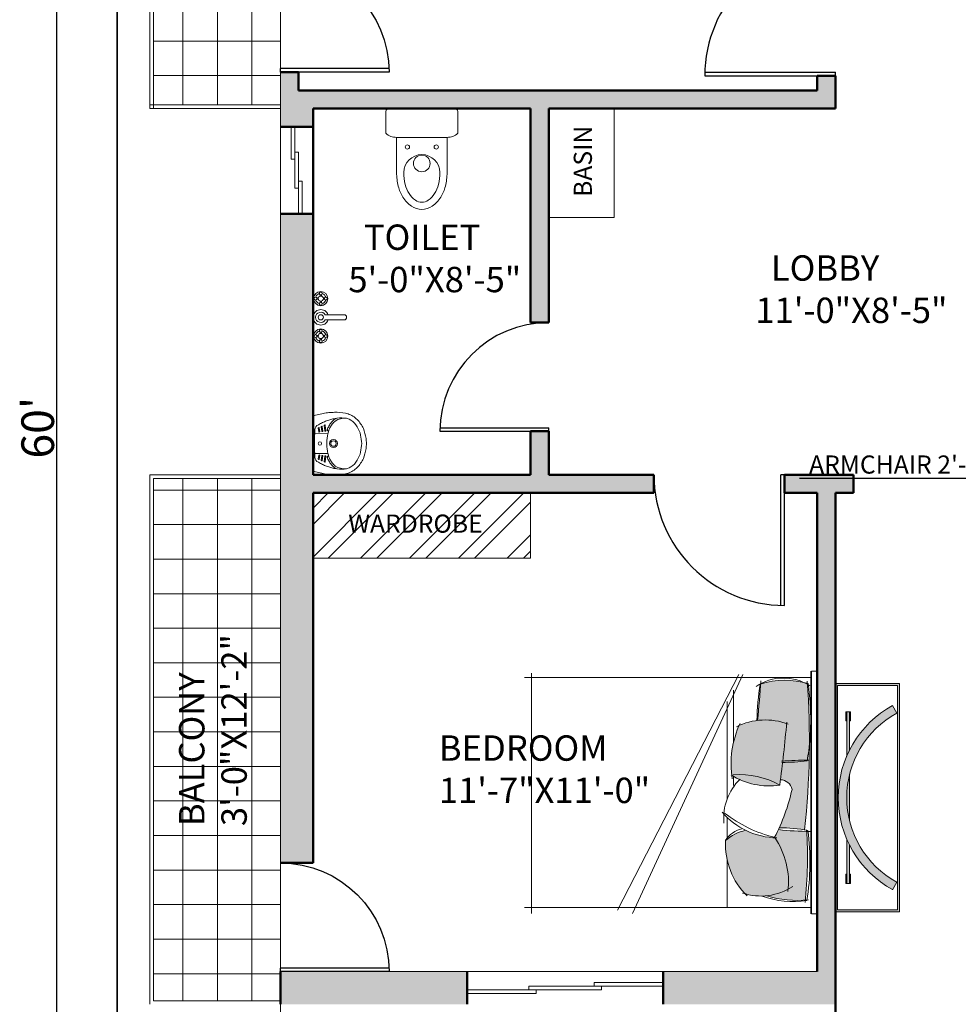
# Model space of a CAD drawing. Units: inches. Extents: x 1734 to 4011, y 1071 to 1891.
# Tile 25 of 27: x 3583 to 3842, y 1313 to 1584. Entities that reach past the tile are written whole.
import ezdxf

# ---------------------------------------------------------------- set-up
doc = ezdxf.new("R2010")
doc.units = ezdxf.units.IN
for name, color, linetype, lineweight in [('0.10', 252, 'Continuous', 9), ('0.15', 34, 'Continuous', 15), ('A-ANNO-DIMS', 2, 'Continuous', 18), ('A-AREA-IDEN', 3, 'Continuous', 18), ('A-DOOR', 3, 'Continuous', 25), ('A-FLOR-FIXT', 9, 'Continuous', 18), ('A-FLOR-PATT', 252, 'Continuous', 13), ('A-FURN', 8, 'Continuous', 18), ('A-FURN-PATT', 252, 'Continuous', 13), ('A-GLAZ', 4, 'Continuous', 18), ('A-WALL', 7, 'Continuous', 50), ('A-WALL-PATT', 8, 'Continuous', 13), ('aparador', 36, 'Continuous', 9), ('C-PROP', 1, 'Continuous', 35), ('moveis', 254, 'Continuous', 5)]:
    doc.layers.add(name, color=color, linetype=linetype, lineweight=lineweight)
doc.styles.get("Standard").update_dxf_attribs({"font": 'arial.ttf'})
doc.dimstyles.new('ISO-25', dxfattribs={"dimtxt": 5, "dimasz": 2.5, "dimexe": 1.25, "dimexo": 0.625, "dimtad": 1, "dimdec": 1, "dimlunit": 3, "dimtxsty": 'Standard', "dimcen": 2.5, "dimclrt": 1, "dimadec": 0, "dimazin": 0, "dimtfac": 1, "dimtdec": 1, "dimtmove": 0, "dimatfit": 3, "dimfxl": 1, "dimarcsym": 0})
pattern_1 = [(90, (598.983, -12.241), (-9.525, 0), []), (180, (598.983, -12.241), (-9e-16, -9.525), [])]

# ---------------------------------------------------------------- blocks, each defined once
blk = doc.blocks.new('*D59')
at = {"layer": 'A-ANNO-DIMS', "color": 0, "lineweight": -2, "transparency": 16777216}
for p, q in [((3609.2, 1831.82), (3591.89, 1831.82)), ((3593.14, 1829.32), (3593.14, 1114.32)), ((3609.2, 1111.82), (3591.89, 1111.82))]:
    blk.add_line(p, q, dxfattribs=at)
at = {"layer": 'A-ANNO-DIMS', "color": 0, "transparency": 16777216}
for points in [[(3592.73, 1829.32), (3593.56, 1829.32), (3593.14, 1831.82)], [(3592.73, 1114.32), (3593.56, 1114.32), (3593.14, 1111.82)]]:
    blk.add_solid(points, dxfattribs=at)
at = {"layer": 'Defpoints', "color": 0, "transparency": 16777216}
for p in [(3609.83, 1831.82), (3593.14, 1111.82), (3609.83, 1111.82)]:
    blk.add_point(p, dxfattribs=at)
at = {"layer": 'A-ANNO-DIMS', "color": 0, "transparency": 16777216, "insert": (3587.92, 1471.82), "char_height": 5, "attachment_point": 5, "rotation": 90}
blk.add_mtext("{\\H1.8x;60'}", dxfattribs=at)
blk = doc.blocks.new("D1 3'")
for p, q in [((0, 36), (0, 0)), ((1, 36), (1, 0)), ((0, 0), (1, 0))]:
    blk.add_line(p, q)
blk.add_arc((0, 0), 36, 0, 90)
blk = doc.blocks.new("D2 2'6")
for p, q in [((0, 30), (0, 0)), ((1, 30), (1, 0)), ((0, 0), (1, 0))]:
    blk.add_line(p, q)
blk.add_arc((0, 0), 30, 0, 90)
blk = doc.blocks.new('camita')
at = {"layer": '0.10'}
for p, q in [((-0.85, -0.045), (0.85, -0.045)), ((-0.805, -0.045), (-0.805, -2.0485)), ((0.805, -0.045), (0.805, -2.0485)), ((-0.8271, -0.521), (0.8464, -1.2932)), ((-0.8271, -0.5476), (0.8236, -1.3992)), ((-0.7161, -0.585), (-0.3554, -0.585)), ((-0.1136, -0.585), (-0.0485, -0.585)), ((-0.638, -0.63), (0.0434, -0.63)), ((0.1749, -0.63), (0.3179, -0.63)), ((0.4739, -0.63), (0.805, -0.63)), ((-0.8354, -2), (0.8464, -2))]:
    blk.add_line(p, q, dxfattribs=at)
blk.add_lwpolyline([(-0.85, -0.0405), (0.85, -0.0405), (0.85, 0), (-0.85, 0)], close=True, dxfattribs=at)
for centre, radius, start, end in [((-0.4574, -0.2364), 0.3443, 147.50996, 213.83359), ((-0.1997, -0.2266), 0.5864, 163.92635, 197.14087), ((-0.3639, -5.8457), 5.7909, 83.80731, 94.12107), ((-0.5104, -1.7232), 1.6781, 80.12554, 98.66187), ((2.3534, -0.0532), 2.5803, 180.10628, 184.38541), ((1.5815, -0.2893), 1.3353, 170.38021, 178.99138), ((-1.4396, -0.0609), 1.7117, 352.92911, 0.39592), ((0.4524, -3.0675), 2.9996, 83.90257, 93.67595), ((0.4863, -1.6286), 1.5781, 80.16015, 98.05996), ((0.0294, -0.1377), 0.7262, 342.58415, 6.00484), ((-1.5443, -0.2452), 1.3333, 359.93941, 7.55329), ((0.1326, -0.1696), 0.6307, 339.92303, 8.74334), ((-0.0543, -0.3633), 0.4542, 159.30257, 206.50263), ((-0.007, -0.258), 0.0828, 100.01798, 179.73597), ((-0.2931, -1.4378), 1.2903, 61.97485, 77.84351), ((0.6265, -0.7518), 0.5508, 82.96906, 124.67388), ((0.3203, -0.3944), 0.4043, 341.45245, 33.45121), ((-1.3301, -9.6748), 9.4985, 82.27078, 84.93989), ((0.4585, -0.5454), 0.5842, 151.04555, 184.14969), ((-0.5341, -0.3393), 0.4875, 327.26442, 9.0473), ((-0.1986, -0.2742), 0.5159, 310.73945, 359.05759), ((-0.5673, -0.0868), 0.9057, 321.69527, 346.46261), ((-1.8672, -14.986), 14.6323, 84.65974, 85.75157), ((-0.4598, 1.4861), 1.9092, 260.95299, 268.65169), ((-0.2002, 0.064), 0.6673, 244.78094, 279.06058), ((0.179, -0.272), 0.3828, 224.52836, 275.22287), ((0.4384, -0.4834), 0.1898, 193.68485, 236.70352), ((0.5707, -0.4317), 0.3145, 192.93877, 221.96363), ((0.3612, -0.133), 0.5096, 267.25889, 315.29965)]:
    blk.add_arc(centre, radius, start, end, dxfattribs=at)
blk = doc.blocks.new('Aparador ORGANICA Formatto')
at = {"layer": 'aparador', "ltscale": 0.3}
h = blk.add_hatch(color=256, dxfattribs=at)
h.dxf.hatch_style = 1
h.set_gradient(color1=(118, 213, 123), color2=(52, 168, 57), one_color=1, tint=0.43, name='INVCURVED')
h.paths.add_polyline_path([(0.8, 0.45), (-0.8, 0.45), (-0.8, 0), (0.8, 0)])
h.paths.add_polyline_path([(0.785, 0.435), (0.785, 0.015), (-0.785, 0.015), (-0.785, 0.435)], flags=16)
h.paths.add_polyline_path([(0.2911, 0.3699), (0.5365, 0.3699), (0.5365, 0.3757), (0.6011, 0.3757), (0.6011, 0.3699), (0.6011, 0.3499), (0.6011, 0.3441), (0.5365, 0.3441), (0.5365, 0.3499), (0.3338, 0.3499, -0.150336), (0.6449, 0.0488), (0.5923, 0.0199, 0.208852), (0.1632, 0.3499), (-0.1632, 0.3499, 0.208852), (-0.5923, 0.0199), (-0.6449, 0.0488, -0.150336), (-0.3338, 0.3499), (-0.5365, 0.3499), (-0.5365, 0.3441), (-0.6011, 0.3441), (-0.6011, 0.3499), (-0.6011, 0.3699), (-0.6011, 0.3757), (-0.5365, 0.3757), (-0.5365, 0.3699), (-0.2911, 0.3699, -0.206106)], flags=0)
h = blk.add_hatch(color=256, dxfattribs=at)
h.dxf.hatch_style = 1
h.set_gradient(color1=(135, 92, 69), color2=(0, 0, 0), one_color=1, name='INVCURVED')
h.paths.add_polyline_path([(-0.6449, 0.0488), (-0.5923, 0.0199, -0.590888), (0.5923, 0.0199), (0.6449, 0.0488, 0.590888)])
h = blk.add_hatch(color=256, dxfattribs=at)
h.dxf.hatch_style = 1
h.set_gradient(color1=(178, 189, 189), one_color=1, tint=1, name='CYLINDER')
h.paths.add_polyline_path([(-0.5365, 0.3757), (-0.6011, 0.3757), (-0.6011, 0.3699), (-0.5365, 0.3699)])
h.paths.add_polyline_path([(-0.5365, 0.3499), (-0.6011, 0.3499), (-0.6011, 0.3441), (-0.5365, 0.3441)])
h = blk.add_hatch(color=256, dxfattribs=at)
h.dxf.hatch_style = 1
h.set_gradient(color1=(118, 213, 123), color2=(31, 101, 35), one_color=1, tint=0.26, name='INVCURVED')
h.paths.add_polyline_path([(-0.2911, 0.3699), (-0.6011, 0.3699), (-0.6011, 0.3499), (-0.3338, 0.3499, -0.015999)])
h = blk.add_hatch(color=256, dxfattribs=at)
h.dxf.hatch_style = 1
h.set_gradient(color1=(118, 213, 123), color2=(31, 101, 35), one_color=1, tint=0.26, name='INVCURVED')
h.paths.add_polyline_path([(-0.1632, 0.3499), (0.1632, 0.3499, 0.122516)])
h = blk.add_hatch(color=256, dxfattribs=at)
h.dxf.hatch_style = 1
h.set_gradient(color1=(118, 213, 123), color2=(31, 101, 35), one_color=1, tint=0.26, name='INVCURVED')
h.paths.add_polyline_path([(0.6011, 0.3699), (0.2911, 0.3699, -0.015999), (0.3338, 0.3499), (0.6011, 0.3499)])
h = blk.add_hatch(color=256, dxfattribs=at)
h.dxf.hatch_style = 1
h.set_gradient(color1=(178, 189, 189), one_color=1, tint=1, name='CYLINDER')
h.paths.add_polyline_path([(0.6011, 0.3757), (0.5365, 0.3757), (0.5365, 0.3699), (0.6011, 0.3699)])
h.paths.add_polyline_path([(0.6011, 0.3499), (0.5365, 0.3499), (0.5365, 0.3441), (0.6011, 0.3441)])
for p, q in [((-0.5923, 0.0199), (-0.6449, 0.0488)), ((0.5923, 0.0199), (0.6449, 0.0488))]:
    blk.add_line(p, q, dxfattribs=at)
for points in [[(-0.6011, 0.3699), (-0.6011, 0.3757), (-0.5365, 0.3757), (-0.5365, 0.3699)], [(-0.5365, 0.3499), (-0.5365, 0.3441), (-0.6011, 0.3441), (-0.6011, 0.3499)], [(0.6011, 0.3699), (0.6011, 0.3757), (0.5365, 0.3757), (0.5365, 0.3699)], [(0.5365, 0.3499), (0.5365, 0.3441), (0.6011, 0.3441), (0.6011, 0.3499)]]:
    blk.add_lwpolyline(points, dxfattribs=at)
for radius in [0.7362, 0.6762]:
    blk.add_arc((0, -0.3063), radius, 28.84335, 151.15665, dxfattribs=at)
at = {"layer": 'moveis', "ltscale": 0.3}
for p, q in [((-0.6011, 0.3699), (-0.6011, 0.3499)), ((-0.2911, 0.3699), (-0.6011, 0.3699)), ((-0.6011, 0.3499), (-0.3338, 0.3499)), ((-0.1632, 0.3499), (0.1632, 0.3499)), ((0.2911, 0.3699), (0.6011, 0.3699)), ((0.6011, 0.3499), (0.3338, 0.3499)), ((0.6011, 0.3699), (0.6011, 0.3499))]:
    blk.add_line(p, q, dxfattribs=at)
for points in [[(-0.8, 0), (0.8, 0), (0.8, 0.45), (-0.8, 0.45)], [(-0.785, 0.015), (0.785, 0.015), (0.785, 0.435), (-0.785, 0.435)]]:
    blk.add_lwpolyline(points, close=True, dxfattribs=at)
blk = doc.blocks.new('Faucet - Bathroom top')
for p, q in [((-4.107, 0.125), (-4.375, 0.125)), ((-3.75, 0.4788), (-3.75, 0.75)), ((-3.5, 0.482), (-3.5, 0.75)), ((-3.1461, 0.125), (-2.875, 0.125)), ((3.143, 0.125), (2.875, 0.125)), ((3.5, 0.4788), (3.5, 0.75)), ((3.75, 0.482), (3.75, 0.75)), ((4.1039, 0.125), (4.375, 0.125)), ((-4.1039, -0.125), (-4.375, -0.125)), ((-3.75, -0.4821), (-3.75, -0.75)), ((-3.5, -0.4789), (-3.5, -0.75)), ((-3.143, -0.125), (-2.875, -0.125)), ((-0.5, -0.8639), (-0.5, -4.5)), ((0.5, -4.5), (0.5, -0.8631)), ((3.1461, -0.125), (2.875, -0.125)), ((3.5, -0.4821), (3.5, -0.75)), ((3.75, -0.4789), (3.75, -0.75)), ((4.107, -0.125), (4.375, -0.125))]:
    blk.add_line(p, q)
for centre, radius in [((-3.625, 0), 1.375), ((-4.625, 0), 0.2795), ((-3.625, 0), 0.5), ((-3.625, 1), 0.2795), ((-2.625, 0), 0.2795), ((0, 0), 0.5), ((3.625, 0), 1.375), ((2.625, 0), 0.2795), ((3.625, 0), 0.5), ((3.625, 1), 0.2795), ((4.625, 0), 0.2795), ((-3.625, -1), 0.2795), ((3.625, -1), 0.2795)]:
    blk.add_circle(centre, radius)
for centre, radius, start, end in [((-3.625, 0), 1, 105.2407, 164.2093), ((-3.625, 0), 1, 16.44125, 74.07887), ((0, 0), 1.5, 289.6514, 250.3603), ((0, 0), 1, 300.3431, 239.7554), ((3.625, 0), 1, 106.12, 164.0884), ((3.625, 0), 1, 16.23422, 73.90469), ((-3.625, 0), 1, 196.2342, 253.9047), ((-3.625, 0), 1, 286.12, 344.0884), ((3.625, 0), 1, 196.4413, 254.0789), ((3.625, 0), 1, 285.2407, 344.2093), ((0, -4.5), 0.5, 180, 0)]:
    blk.add_arc(centre, radius, start, end)
blk = doc.blocks.new('lavamanos 2')
at = {"layer": '0.15'}
for p, q in [((0, 0.2335), (0, -0.2335)), ((-0.1304, 0.11), (-0.1315, 0.11)), ((-0.0142, 0.087), (-0.13, 0.086)), ((-0.1127, 0.112), (-0.1067, 0.1581)), ((-0.1037, 0.1109), (-0.0978, 0.157)), ((-0.0857, 0.1085), (-0.0807, 0.1466)), ((-0.0767, 0.1074), (-0.0718, 0.1455)), ((-0.0587, 0.105), (-0.0548, 0.1351)), ((-0.0497, 0.1039), (-0.0458, 0.134)), ((-0.1304, -0.11), (-0.1315, -0.11)), ((-0.0142, -0.087), (-0.13, -0.086)), ((-0.1127, -0.112), (-0.1067, -0.1581)), ((-0.1037, -0.1109), (-0.0978, -0.157)), ((-0.0857, -0.1085), (-0.0807, -0.1466)), ((-0.0767, -0.1074), (-0.0718, -0.1455)), ((-0.0587, -0.105), (-0.0548, -0.1351)), ((-0.0497, -0.1039), (-0.0458, -0.134))]:
    blk.add_line(p, q, dxfattribs=at)
for centre, radius in [((-0.178, 0), 0.035), ((-0.178, 0), 0.0235), ((-0.06, 0), 0.015)]:
    blk.add_circle(centre, radius, dxfattribs=at)
for centre, radius, start, end in [((-0.2419, 0.0663), 0.2023, 108.1945, 135.36859), ((-0.2035, -0.0862), 0.3593, 91.20299, 106.42552), ((-0.2208, -0.6855), 0.9585, 86.55138, 89.41308), ((-0.2121, -0.5476), 0.8204, 83.12241, 86.5796), ((5.8279, 30.215), 30.5319, 258.77821, 258.87599), ((-0.1663, 0.0005), 0.3024, 136.57187, 154.32772), ((-0.2422, 0.0655), 0.1638, 121.99295, 150.58892), ((-0.2657, 0.1037), 0.119, 92.47742, 122.14108), ((-0.2765, 0.0677), 0.1528, 57.2491, 95.54005), ((-0.2442, -0.0128), 0.2368, 77.24819, 96.46321), ((-0.2765, 0.0677), 0.1678, 56.87663, 64.99714), ((-0.3662, -0.002), 0.2627, 40.35252, 49.00458), ((-0.2222, 0.0026), 0.2177, 71.98488, 82.01242), ((-0.3662, -0.002), 0.2777, 40.35252, 49.22548), ((-0.3103, -0.315), 0.5472, 69.51913, 73.49118), ((-0.2374, 0.11), 0.1071, 27.57433, 39.11562), ((-0.2991, -0.2855), 0.5156, 65.23004, 69.53785), ((-0.2784, -0.2408), 0.4663, 60.24131, 65.2382), ((-0.1265, -0.0657), 0.3287, 69.06009, 78.82181), ((-0.0202, 0.212), 0.0314, 54.79491, 69.06009), ((-0.005, 0.2335), 0.005, 0, 54.79491), ((-0.0557, -0.0178), 0.4111, 158.70106, 171.31016), ((-0.1999, 0.0263), 0.2202, 147.11565, 167.44248), ((-0.2374, 0.11), 0.0921, 27.31862, 39.11562), ((-0.3494, 0.0363), 0.2258, 22.33605, 30.8927), ((-0.3494, 0.0363), 0.2408, 22.19214, 30.78376), ((-1.2664, -0.2389), 1.1824, 16.36313, 17.77674), ((-0.1315, 0.117), 0.007, 197.40991, 270.49494), ((0.1853, 0.1648), 0.325, 192.53887, 196.70718), ((-0.1305, 0.117), 0.007, 270.49494, 17.39527), ((-1.2664, -0.2389), 1.1974, 17.39527, 17.80495), ((-0.1082, 0.1115), 0.0045, 172.61396, 352.61396), ((-0.1022, 0.1575), 0.0045, 352.61396, 172.61396), ((-0.0812, 0.108), 0.0045, 172.61396, 352.61396), ((-0.0763, 0.146), 0.0045, 352.61396, 172.61396), ((-0.0542, 0.1045), 0.0045, 172.61396, 352.61396), ((-0.0503, 0.1345), 0.0045, 352.61396, 172.61396), ((-0.0648, 0.1184), 0.049, 1.58272, 68.62081), ((-2.1477, 0.0009), 2.1352, 359.97535, 3.19009), ((-0.2093, 0.0056), 0.2558, 171.31016, 181.26266), ((-0.2093, -0.0056), 0.2558, 178.73734, 188.68984), ((0.4664, -0.0834), 0.8953, 169.86317, 174.65802), ((0.4664, 0.0834), 0.8953, 185.34198, 190.13683), ((0.3887, 0.121), 0.517, 185.50529, 189.81306), ((-0.7181, -0.0071), 0.5987, 0.67647, 3.82165), ((-0.7181, 0.0071), 0.5987, 356.17835, 359.32353), ((-2.1477, -0.0009), 2.1352, 356.80991, 0.02465), ((-0.0557, 0.0178), 0.4111, 188.68984, 201.29894), ((-0.1999, -0.0263), 0.2202, 192.55752, 212.88435), ((0.1853, -0.1648), 0.325, 163.29282, 167.46113), ((0.3887, -0.1209), 0.517, 170.18694, 174.49471), ((-0.1663, -0.0005), 0.3024, 205.67228, 223.42813), ((-0.2422, -0.0655), 0.1638, 209.41108, 238.00705), ((-0.3662, 0.002), 0.2627, 310.99542, 319.64748), ((-0.2374, -0.1099), 0.0921, 320.88438, 332.68138), ((-0.3494, -0.0363), 0.2258, 329.1073, 337.66395), ((-0.2374, -0.1099), 0.1071, 320.88438, 332.42567), ((-0.3494, -0.0363), 0.2408, 329.21624, 337.80786), ((-1.2664, 0.2389), 1.1824, 342.22326, 343.63687), ((-0.1315, -0.117), 0.007, 89.50506, 162.59009), ((-0.1305, -0.117), 0.007, 342.60473, 89.50506), ((-1.2664, 0.2389), 1.1974, 342.19505, 342.60473), ((-0.1082, -0.1115), 0.0045, 7.38604, 187.38604), ((-0.1022, -0.1575), 0.0045, 187.38604, 7.38604), ((-0.0812, -0.108), 0.0045, 7.38604, 187.38604), ((-0.2784, 0.2408), 0.4663, 294.7618, 299.75869), ((-0.0763, -0.146), 0.0045, 187.38604, 7.38604), ((-0.0542, -0.1045), 0.0045, 7.38604, 187.38604), ((-0.0503, -0.1345), 0.0045, 187.38604, 7.38604), ((-0.0648, -0.1184), 0.049, 291.37919, 358.41728), ((-0.2419, -0.0663), 0.2023, 224.63141, 251.8055), ((-0.2657, -0.1036), 0.119, 237.85892, 267.52258), ((-0.2765, -0.0677), 0.1528, 264.45995, 302.7509), ((-0.2442, 0.0128), 0.2368, 263.53679, 282.75181), ((-0.2765, -0.0677), 0.1678, 295.00286, 303.12337), ((-0.2222, -0.0026), 0.2177, 277.98758, 288.01512), ((-0.3662, 0.002), 0.2777, 310.77452, 319.64748), ((-0.3103, 0.315), 0.5472, 286.50882, 290.48087), ((-0.2991, 0.2855), 0.5156, 290.46215, 294.76996), ((5.8279, -30.215), 30.5319, 101.12401, 101.22179), ((-0.1265, 0.0657), 0.3287, 281.17819, 290.93991), ((-0.0202, -0.212), 0.0314, 290.93991, 305.20509), ((-0.005, -0.2335), 0.005, 305.20509, 0), ((-0.2035, 0.0862), 0.3593, 253.57448, 268.79701), ((-0.2208, 0.6855), 0.9585, 270.58692, 273.44862), ((-0.2121, 0.5476), 0.8204, 273.4204, 276.87759)]:
    blk.add_arc(centre, radius, start, end, dxfattribs=at)
blk = doc.blocks.new('rreerr')
blk.add_lwpolyline([(2512.8529, 833.5601, 0.205217), (2512.9279, 833.5883), (2512.9279, 833.7401, 0.414214), (2512.9079, 833.7601), (2512.4479, 833.7601, 0.414214), (2512.4279, 833.7401), (2512.4279, 833.5883, 0.205217), (2512.5029, 833.5601)], format="xyb")
for points in [[(2512.5468, 833.1438, 0.107027), (2512.6056, 833.0819, 0.150548), (2512.6779, 833.0596, 0.150548), (2512.7502, 833.0819, 0.107027), (2512.809, 833.1438, 0.075071), (2512.8412, 833.2206, 0.0618), (2512.8529, 833.3151), (2512.8529, 833.5601), (2512.5029, 833.5601), (2512.5029, 833.3151, 0.0618), (2512.5146, 833.2206, 0.075071)], [(2512.5631, 833.2328, 0.075071), (2512.5895, 833.1698, 0.107027), (2512.6338, 833.1232, 0.150548), (2512.6779, 833.1096, 0.150548), (2512.722, 833.1232, 0.107027), (2512.7663, 833.1698, 0.075071), (2512.7927, 833.2328, 0.0618), (2512.8029, 833.3151, 1), (2512.5529, 833.3151, 0.0618)]]:
    blk.add_lwpolyline(points, format="xyb", close=True)
for centre, radius in [((2512.5779, 833.493), 0.0146), ((2512.7779, 833.493), 0.0146), ((2512.6775, 833.3793), 0.0579)]:
    blk.add_circle(centre, radius)
blk = doc.blocks.new('*D87')
at = {"layer": 'A-ANNO-DIMS', "color": 0, "lineweight": -2, "transparency": 16777216}
for p, q in [((3871.63, 1454.4), (3871.63, 1459.05)), ((3898.44, 1454.4), (3898.44, 1459.05)), ((3871.63, 1457.8), (3797.91, 1457.8)), ((3895.94, 1457.8), (3874.13, 1457.8))]:
    blk.add_line(p, q, dxfattribs=at)
at = {"layer": 'A-ANNO-DIMS', "color": 0, "transparency": 16777216}
for points in [[(3874.13, 1458.22), (3874.13, 1457.38), (3871.63, 1457.8)], [(3895.94, 1458.22), (3895.94, 1457.38), (3898.44, 1457.8)]]:
    blk.add_solid(points, dxfattribs=at)
at = {"layer": 'Defpoints', "color": 0, "transparency": 16777216}
for p in [(3871.63, 1457.8), (3871.63, 1453.78), (3898.44, 1453.78)]:
    blk.add_point(p, dxfattribs=at)
at = {"layer": 'A-ANNO-DIMS', "color": 1, "transparency": 16777216, "insert": (3833.52, 1461.01), "char_height": 5, "attachment_point": 5}
blk.add_mtext('ARMCHAIR 2\'-3" TYP.', dxfattribs=at)

msp = doc.modelspace()

# ---------------------------------------------------------------- hatches: boundary and pattern name
at = {"layer": 'A-FLOR-PATT'}
h = msp.add_hatch(dxfattribs=at)
h.set_pattern_fill('ANSI37', color=256, scale=3, angle=45)
h.set_pattern_definition(pattern_1)
h.paths.add_polyline_path([(3654.83, 1745.82), (3619.83, 1745.82), (3619.83, 1560.82), (3654.83, 1560.82), (3654.83, 1569.82), (3654.83, 1570.82)])
h.paths.add_polyline_path([(3649.53, 1630.8), (3649.53, 1685.51), (3623.41, 1685.51), (3623.41, 1630.8)], flags=24)
h = msp.add_hatch(dxfattribs=at)
h.set_pattern_fill('ANSI37', color=256, scale=3, angle=45)
h.set_pattern_definition(pattern_1)
h.paths.add_polyline_path([(3619.83, 1313.82), (3654.83, 1313.82), (3654.83, 1457.82), (3619.83, 1457.82)])
h.paths.add_polyline_path([(3649.53, 1359.49), (3649.53, 1414.2), (3623.41, 1414.2), (3623.41, 1359.49)], flags=24)
h = msp.add_hatch(dxfattribs=at)
h.set_pattern_fill('ANSI37', color=256, scale=3, angle=45)
h.set_pattern_definition(pattern_1)
h.paths.add_polyline_path([(3619.83, 1313.82), (3654.83, 1313.82), (3654.83, 1457.82), (3619.83, 1457.82)])
h.paths.add_polyline_path([(3649.53, 1359.49), (3649.53, 1414.2), (3623.41, 1414.2), (3623.41, 1359.49)], flags=24)
at = {"layer": 'A-FURN-PATT'}
h = msp.add_hatch(dxfattribs=at)
h.set_pattern_fill('ANSI32', color=256)
h.set_pattern_definition([(45, (598.983, -12.241), (-6.735192, 6.735192), []), (45, (603.473, -12.241), (-6.735192, 6.735192), [])])
h.paths.add_polyline_path([(3723.83, 1453.82), (3663.83, 1453.82), (3663.83, 1435.82), (3723.83, 1435.82)])
h.paths.add_polyline_path([(3667.71, 1440.04), (3717.17, 1440.04), (3717.17, 1450.34), (3667.71, 1450.34)], flags=24)
h.paths.add_polyline_path([(3882.46, 1633.93), (3882.46, 1688.64), (3856.34, 1688.64), (3856.34, 1633.93)], flags=9)
h.paths.add_polyline_path([(3912.44, 1633.93), (3912.44, 1688.64), (3886.32, 1688.64), (3886.32, 1633.93)], flags=9)
h.paths.add_polyline_path([(3849.42, 1795.58), (3903.83, 1795.58), (3903.83, 1821.7), (3849.42, 1821.7)], flags=9)
h.paths.add_polyline_path([(3821.75, 1770.76), (3864.43, 1770.76), (3864.43, 1779), (3821.75, 1779)], flags=9)
h.paths.add_polyline_path([(3824.93, 1134.29), (3837.52, 1134.29), (3837.52, 1144.59), (3824.93, 1144.59)], flags=9)
h.paths.add_polyline_path([(3824.92, 1203.29), (3837.13, 1203.29), (3837.13, 1213.59), (3824.92, 1213.59)], flags=9)
h.paths.add_polyline_path([(3649.53, 1633.93), (3649.53, 1688.64), (3623.41, 1688.64), (3623.41, 1633.93)], flags=9)
h.paths.add_polyline_path([(3861.96, 1555.4), (3916.37, 1555.4), (3916.37, 1581.52), (3861.96, 1581.52)], flags=9)
h.paths.add_polyline_path([(3920.06, 1601.91), (3940.42, 1601.91), (3940.42, 1612.21), (3920.06, 1612.21)], flags=9)
h.paths.add_polyline_path([(3879.75, 1638.04), (3929.21, 1638.04), (3929.21, 1648.34), (3879.75, 1648.34)], flags=9)
h.paths.add_polyline_path([(3861.7, 1695.43), (3921.55, 1695.43), (3921.55, 1721.55), (3861.7, 1721.55)], flags=9)
h.paths.add_polyline_path([(3738.69, 1778.27), (3787.65, 1778.27), (3787.65, 1804.39), (3738.69, 1804.39)], flags=9)
h.paths.add_polyline_path([(3649.33, 1778.26), (3698.3, 1778.26), (3698.3, 1804.38), (3649.33, 1804.38)], flags=9)
h.paths.add_polyline_path([(3687.88, 1211.9), (3747.72, 1211.9), (3747.72, 1238.02), (3687.88, 1238.02)], flags=9)
h.paths.add_polyline_path([(3782.95, 1496.7), (3837.36, 1496.7), (3837.36, 1522.82), (3782.95, 1522.82)], flags=9)
h.paths.add_polyline_path([(3862.83, 1344.86), (3931.88, 1344.86), (3931.88, 1370.98), (3862.83, 1370.98)], flags=9)
h.paths.add_polyline_path([(3887.8, 1472.31), (3942.21, 1472.31), (3942.21, 1498.43), (3887.8, 1498.43)], flags=9)
h.paths.add_polyline_path([(3707.14, 1647.71), (3772.42, 1647.71), (3772.42, 1673.83), (3707.14, 1673.83)], flags=9)
h = msp.add_hatch(color=256, dxfattribs=at)
h.dxf.hatch_style = 1
h.paths.add_polyline_path([(3800.14, 1401.05, 0.020657), (3799.14, 1401.56, 0.131047), (3787.25, 1401.18, -0.004387), (3786.4, 1391.11, -0.113891), (3794.39, 1390.24, -0.006967), (3793.32, 1379.88, -0.016701), (3800.1, 1380.15, 0.015442), (3800.67, 1384.19, 0.01851)])
h.paths.add_polyline_path([(3794.39, 1390.24, 0.189536), (3781.32, 1389.72, 0.134508), (3779.25, 1375.99, 0.181694), (3792.49, 1373.29, 0.011408)])
h.paths.add_polyline_path([(3791.16, 1358.74, -0.104045), (3783.05, 1360.81, 0.127326), (3777.54, 1357.95, 0.202559), (3782.93, 1343.29, 0.194952), (3794.82, 1344.57, 0.173835)])
h.paths.add_polyline_path([(3799.94, 1360.5, -0.029051), (3792.13, 1361.01, -0.011742), (3791.06, 1358.88, -0.175864), (3794.82, 1344.57, -0.098488), (3788.88, 1342.76, 0.094792), (3799.55, 1341.54, 0.040212)])
h = msp.add_hatch(color=256, dxfattribs=at)
h.dxf.hatch_style = 1
h.paths.add_polyline_path([(3792.36, 1361.51, -0.033321), (3799.34, 1360.92, 0.021136), (3800.61, 1380.15, 0.017944), (3793.32, 1379.88, -0.003455), (3792.68, 1374.75, -0.362577), (3795.88, 1372.05, -0.054862)])
at = {"layer": 'A-WALL-PATT'}
h = msp.add_hatch(color=256, dxfattribs=at)
h.dxf.hatch_style = 1
h.paths.add_polyline_path([(3663.83, 1530.82), (3654.83, 1530.82), (3654.83, 1351.82), (3663.83, 1351.82), (3663.83, 1453.82), (3757.83, 1453.82), (3757.83, 1458.82), (3728.83, 1458.82), (3728.83, 1470.82), (3723.83, 1470.82), (3723.83, 1458.82), (3663.83, 1458.82)])
h.paths.add_polyline_path([(3706.33, 1321.82), (3654.83, 1321.82), (3654.83, 1312.82), (3706.33, 1312.82)])
h.paths.add_polyline_path([(3807.83, 1453.82), (3812.83, 1453.82), (3812.83, 1458.82), (3793.83, 1458.82), (3793.83, 1453.82), (3802.83, 1453.82), (3802.83, 1321.82), (3760.33, 1321.82), (3760.33, 1312.82), (3807.83, 1312.82)])
h.paths.add_polyline_path([(3807.83, 1288.82), (3798.83, 1288.82), (3798.83, 1285.82), (3807.83, 1285.82)])
h.paths.add_polyline_path([(3807.83, 1568.82), (3802.83, 1568.82), (3802.83, 1564.82), (3659.83, 1564.82), (3659.83, 1569.82), (3654.83, 1569.82), (3654.83, 1554.82), (3663.83, 1554.82), (3663.83, 1559.82), (3723.83, 1559.82), (3723.83, 1500.82), (3728.83, 1500.82), (3728.83, 1559.82), (3807.83, 1559.82)])
h.paths.add_polyline_path([(3659.83, 1623.83), (3654.83, 1623.83), (3654.83, 1599.82), (3659.83, 1599.82)])
h.paths.add_polyline_path([(3720.83, 1750.82), (3651.39, 1750.82), (3651.39, 1745.82), (3654.83, 1745.82), (3654.83, 1671.83), (3659.83, 1671.83), (3659.83, 1745.82), (3720.83, 1745.82)])
h.paths.add_polyline_path([(3818.83, 1237.82), (3798.83, 1237.82), (3798.83, 1228.82), (3818.83, 1228.82)])

# ---------------------------------------------------------------- linework, layer by layer
at = {"layer": 'A-FURN'}
for p, q in [((3618.83, 1559.82), (3618.83, 1831.82)), ((3619.83, 1559.82), (3619.83, 1745.82)), ((3654.83, 1569.82), (3654.83, 1745.82)), ((3654.83, 1111.82), (3654.83, 1569.82)), ((3618.83, 1560.82), (3654.83, 1560.82)), ((3618.83, 1312.82), (3618.83, 1458.82)), ((3618.83, 1458.82), (3654.83, 1458.82)), ((3619.83, 1313.82), (3619.83, 1457.82)), ((3619.83, 1457.82), (3654.83, 1457.82)), ((3663.83, 1435.82), (3723.83, 1435.82)), ((3654.83, 1321.82), (3802.83, 1321.82)), ((3619.83, 1313.82), (3654.83, 1313.82))]:
    msp.add_line(p, q, dxfattribs=at)
at = {"layer": 'A-GLAZ'}
for p, q in [((3618.83, 1559.82), (3654.83, 1559.82)), ((3746.83, 1529.82), (3746.83, 1559.82)), ((3657.83, 1545.82), (3657.83, 1554.82)), ((3658.83, 1537.82), (3658.83, 1554.82)), ((3659.83, 1547.82), (3658.83, 1547.82)), ((3659.83, 1530.82), (3659.83, 1547.82)), ((3658.83, 1545.82), (3657.83, 1545.82)), ((3660.83, 1539.82), (3659.83, 1539.82)), ((3660.83, 1530.82), (3660.83, 1539.82)), ((3659.83, 1537.82), (3658.83, 1537.82)), ((3728.83, 1529.82), (3746.83, 1529.82)), ((3723.83, 1435.82), (3723.83, 1453.82)), ((3706.33, 1316.82), (3743.33, 1316.82)), ((3723.33, 1317.82), (3723.33, 1316.82)), ((3723.33, 1317.82), (3760.33, 1317.82)), ((3725.33, 1316.82), (3725.33, 1315.82)), ((3741.33, 1318.82), (3741.33, 1317.82)), ((3741.33, 1318.82), (3760.33, 1318.82)), ((3743.33, 1317.82), (3743.33, 1316.82)), ((3706.33, 1315.82), (3725.33, 1315.82))]:
    msp.add_line(p, q, dxfattribs=at)
at = {"layer": 'A-WALL'}
for p, q in [((3654.83, 1569.82), (3659.83, 1569.82)), ((3659.83, 1564.82), (3659.83, 1569.82)), ((3802.83, 1568.82), (3807.83, 1568.82)), ((3802.83, 1564.82), (3802.83, 1568.82)), ((3807.83, 1559.82), (3807.83, 1568.82)), ((3659.83, 1564.82), (3802.83, 1564.82)), ((3663.83, 1559.82), (3723.83, 1559.82)), ((3663.83, 1458.82), (3663.83, 1559.82)), ((3723.83, 1500.82), (3723.83, 1559.82)), ((3728.83, 1559.82), (3807.83, 1559.82)), ((3728.83, 1500.82), (3728.83, 1559.82)), ((3663.83, 1554.82), (3654.83, 1554.82)), ((3663.83, 1530.82), (3654.83, 1530.82)), ((3723.83, 1500.82), (3728.83, 1500.82)), ((3723.83, 1470.82), (3728.83, 1470.82)), ((3723.83, 1458.82), (3723.83, 1470.82)), ((3728.83, 1458.82), (3728.83, 1470.82)), ((3663.83, 1458.82), (3723.83, 1458.82)), ((3728.83, 1458.82), (3757.83, 1458.82)), ((3757.83, 1453.82), (3757.83, 1458.82)), ((3793.83, 1458.82), (3812.83, 1458.82)), ((3793.83, 1453.82), (3793.83, 1458.82)), ((3812.83, 1453.82), (3812.83, 1458.82)), ((3663.83, 1453.82), (3757.83, 1453.82)), ((3663.83, 1351.82), (3663.83, 1453.82)), ((3793.83, 1453.82), (3802.83, 1453.82)), ((3802.83, 1321.82), (3802.83, 1453.82)), ((3807.83, 1453.82), (3812.83, 1453.82)), ((3807.83, 1285.82), (3807.83, 1453.82)), ((3654.83, 1351.82), (3663.83, 1351.82)), ((3654.83, 1312.82), (3654.83, 1321.82)), ((3706.33, 1321.82), (3706.33, 1312.82)), ((3760.33, 1321.82), (3760.33, 1312.82))]:
    msp.add_line(p, q, dxfattribs=at)
at = {"layer": 'C-PROP'}
msp.add_lwpolyline([(3785.83, 1111.82), (3609.83, 1111.82), (3609.83, 1831.82), (3969.83, 1831.82), (3969.83, 1111.82), (3785.83, 1111.82)], dxfattribs=at)

# ---------------------------------------------------------------- block references
at = {"layer": 'A-DOOR'}
for name, p, rotation in [("D1 3'", (3807.83, 1568.82), 90), ("D2 2'6", (3728.83, 1470.82), 90.00000000000003), ("D1 3'", (3793.83, 1458.82), 180)]:
    msp.add_blockref(name, p, dxfattribs=dict(at, rotation=rotation))
at = {"layer": 'A-DOOR', "xscale": -1, "rotation": 270}
for p in [(3654.83, 1569.82), (3654.83, 1321.82)]:
    msp.add_blockref("D2 2'6", p, dxfattribs=at)
at = {"layer": 'A-FLOR-FIXT', "xscale": 39.701, "yscale": 39.701, "zscale": 39.701}
msp.add_blockref('rreerr', (-96062, -31541.29), dxfattribs=at)
at = {"layer": 'A-FLOR-FIXT'}
for name, p, xscale, yscale, zscale, rotation in [('Faucet - Bathroom top', (3665.96, 1502.25), 1.424049708253414, 1.424049708253414, 1.424049708253414, 90), ('lavamanos 2', (3663.83, 1467.45), 31.61240364394164, 31.61240364394164, 31.61240364394164, 179.99990349049)]:
    msp.add_blockref(name, p, dxfattribs=dict(at, xscale=xscale, yscale=yscale, zscale=zscale, rotation=rotation))
at = {"layer": 'A-FURN'}
for name, p, xscale, yscale, zscale, rotation in [('camita', (3802.83, 1371.21), 39.375, 39.375, 39.375, 270), ('Aparador ORGANICA Formatto', (3825.54, 1369.82), 39.3701, 39.3701, 39.3701, 90)]:
    msp.add_blockref(name, p, dxfattribs=dict(at, xscale=xscale, yscale=yscale, zscale=zscale, rotation=rotation))

# ---------------------------------------------------------------- texts
at = {"layer": 'A-AREA-IDEN', "attachment_point": 1, "rotation": 90}
for s, insert, char_height in [('BASIN', (3735.71, 1535.45), 5), ('BALCONY\\P3\'-0"X12\'-2"', (3626.89, 1361.95), 7)]:
    msp.add_mtext_dynamic_manual_height_columns(s, width=86.9528, gutter_width=12.5, heights=[0], dxfattribs=dict(at, insert=insert, char_height=char_height))
at = {"layer": 'A-AREA-IDEN', "attachment_point": 1}
for s, insert, char_height in [('  TOILET\\P5\'-0"X8\'-5"', (3673.56, 1527.84), 7), ('  LOBBY\\P11\'-0"X8\'-5"', (3785.77, 1519.35), 7), ('   WARDROBE', (3668.96, 1447.86), 5), ('BEDROOM\\P11\'-7"X11\'-0"', (3698.51, 1386.98), 7)]:
    msp.add_mtext_dynamic_manual_height_columns(s, width=86.9528, gutter_width=12.5, heights=[0], dxfattribs=dict(at, insert=insert, char_height=char_height))

# ---------------------------------------------------------------- dimensions: what is measured, and where the dimension line sits
at = {"layer": 'A-ANNO-DIMS'}
for base, p1, p2, angle, text, override, picture, middle in [((3593.14, 1111.82), (3609.83, 1831.82), (3609.83, 1111.82), 90, '{\\H1.8x;<>}', {"dimclrd": 0, "dimclre": 0, "dimclrt": 0}, '*D59', (3587.92, 1471.82)), ((3871.63, 1457.8), (3898.44, 1453.78), (3871.63, 1453.78), 180, 'ARMCHAIR <> TYP.', {"dimdec": 1, "dimrnd": 0, "dimzin": 1, "dimlunit": 4, "dimfrac": 2}, '*D87', (3833.52, 1461.01))]:
    dim = msp.add_linear_dim(base=base, p1=p1, p2=p2, angle=angle, text=text, dimstyle='ISO-25', override=override, dxfattribs=at)
    dim.commit()
    dim.dimension.update_dxf_attribs({"geometry": picture, "text_midpoint": middle})

doc.saveas('drawing.dxf')
